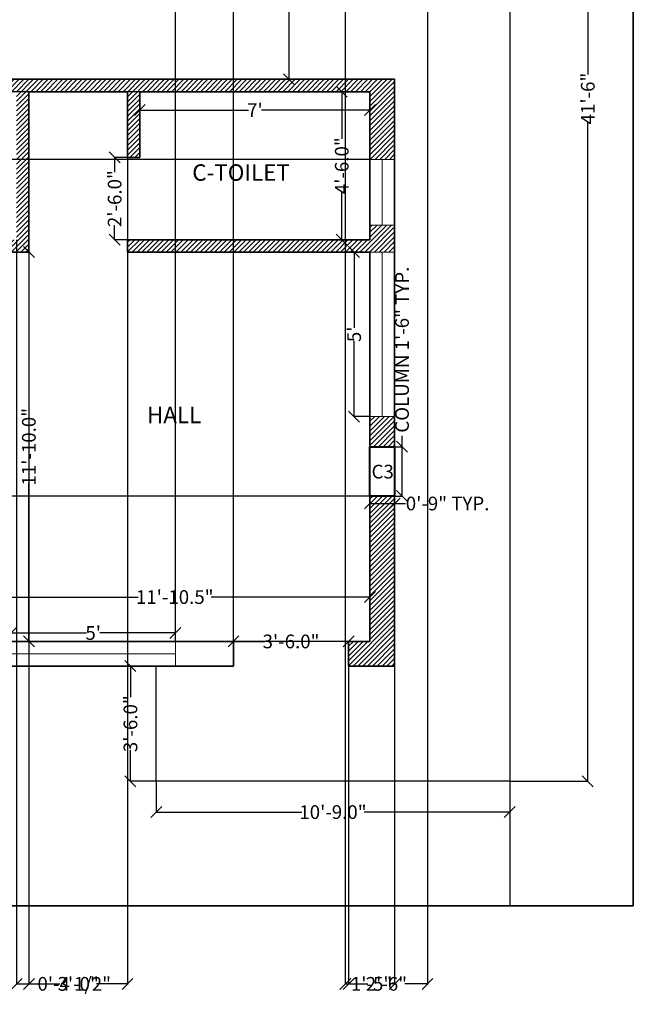
# Model space of a CAD drawing. Units: inches. Extents: x 72 to 538, y -43 to 598.
# Tile 2 of 4: x 314 to 538, y -43 to 316. Entities that reach past the tile are written whole.
import ezdxf

# ---------------------------------------------------------------- set-up
doc = ezdxf.new("R2010")
doc.units = ezdxf.units.IN
doc.header["$MEASUREMENT"] = 0
for name, color, linetype, lineweight in [('A-ANNO-DIMS', 2, 'Continuous', 18), ('A-ANNO-TEXT', 6, 'Continuous', 18), ('A-ANNO-TTLB', 7, 'Continuous', 35), ('A-AREA-IDEN', 7, 'Continuous', 25), ('A-COLS', 6, 'Continuous', 40), ('A-GLAZ', 4, 'Continuous', 18), ('A-WALL', 7, 'Continuous', 35), ('C-SITE', 7, 'Continuous', 25)]:
    doc.layers.add(name, color=color, linetype=linetype, lineweight=lineweight)
doc.layers.add('A-WALL-PATT', color=30, linetype='Continuous', lineweight=13, true_color=0xf26722)
doc.styles.get("Standard").update_dxf_attribs({"font": 'arial.ttf'})
doc.dimstyles.get("Standard").update_dxf_attribs({"dimtxt": 5, "dimasz": 4, "dimexe": 0.18, "dimexo": 0.0625, "dimgap": 0.09, "dimtad": 0, "dimdec": 1, "dimzin": 0, "dimdsep": 46, "dimlunit": 3, "dimtxsty": 'Standard', "dimblk": 'OBLIQUE', "dimcen": 0.09, "dimadec": 0, "dimazin": 0, "dimtfac": 1, "dimtdec": 1, "dimtofl": 0, "dimtmove": 0, "dimatfit": 3, "dimfxl": 1, "dimtolj": 1, "dimtzin": 0, "dimarcsym": 0})

# ---------------------------------------------------------------- blocks, each defined once
blk = doc.blocks.new('_Oblique')
at = {"color": 0, "linetype": 'ByBlock', "lineweight": -2}
blk.add_line((-0.5, -0.5), (0.5, 0.5), dxfattribs=at)
blk = doc.blocks.new('*D20')
at = {"layer": 'A-ANNO-DIMS', "color": 0, "lineweight": -2, "transparency": 16777216}
for p, q in [((317.13, 231.12), (317.13, 173.42)), ((317.19, 231.12), (317.31, 231.12)), ((317.13, 89.12), (317.13, 146.82)), ((317.19, 89.12), (317.31, 89.12))]:
    blk.add_line(p, q, dxfattribs=at)
at = {"layer": 'Defpoints', "color": 0, "transparency": 16777216}
for p in [(317.13, 231.12), (317.13, 89.12), (317.13, 89.12)]:
    blk.add_point(p, dxfattribs=at)
at = {"layer": 'A-ANNO-DIMS', "color": 0, "lineweight": -2, "transparency": 16777216, "xscale": 4, "yscale": 4, "zscale": 4}
for p, rotation in [((317.13, 231.12), 90), ((317.13, 89.12), 270)]:
    blk.add_blockref('_Oblique', p, dxfattribs=dict(at, rotation=rotation))
at = {"layer": 'A-ANNO-DIMS', "color": 0, "transparency": 16777216, "insert": (317.13, 160.12), "char_height": 5, "attachment_point": 5, "rotation": 90}
blk.add_mtext('\\A1;11\'-10.0"', dxfattribs=at)
blk = doc.blocks.new('*D21')
at = {"layer": 'A-ANNO-DIMS', "color": 0, "lineweight": -2, "transparency": 16777216}
for p, q in [((299.13, 113.52), (299.13, 105.13)), ((441.63, 113.52), (441.63, 105.13)), ((299.13, 105.31), (357.08, 105.31)), ((441.63, 105.31), (383.68, 105.31))]:
    blk.add_line(p, q, dxfattribs=at)
at = {"layer": 'Defpoints', "color": 0, "transparency": 16777216}
for p in [(299.13, 113.59), (441.63, 113.59), (441.63, 105.31)]:
    blk.add_point(p, dxfattribs=at)
at = {"layer": 'A-ANNO-DIMS', "color": 0, "lineweight": -2, "transparency": 16777216, "xscale": 4, "yscale": 4, "zscale": 4, "rotation": 180}
blk.add_blockref('_Oblique', (299.13, 105.31), dxfattribs=at)
at = {"layer": 'A-ANNO-DIMS', "color": 0, "lineweight": -2, "transparency": 16777216, "xscale": 4, "yscale": 4, "zscale": 4}
blk.add_blockref('_Oblique', (441.63, 105.31), dxfattribs=at)
at = {"layer": 'A-ANNO-DIMS', "color": 0, "transparency": 16777216, "insert": (370.38, 105.31), "char_height": 5, "attachment_point": 5}
blk.add_mtext('\\A1;11\'-10.5"', dxfattribs=at)
blk = doc.blocks.new('*D22')
at = {"layer": 'A-ANNO-DIMS', "color": 0, "lineweight": -2, "transparency": 16777216}
for p, q in [((441.57, 231.12), (435.66, 231.12)), ((435.84, 231.12), (435.84, 203.51)), ((435.84, 171.12), (435.84, 198.73)), ((441.57, 171.12), (435.66, 171.12))]:
    blk.add_line(p, q, dxfattribs=at)
at = {"layer": 'Defpoints', "color": 0, "transparency": 16777216}
for p in [(441.63, 231.12), (435.84, 171.12), (441.63, 171.12)]:
    blk.add_point(p, dxfattribs=at)
at = {"layer": 'A-ANNO-DIMS', "color": 0, "lineweight": -2, "transparency": 16777216, "xscale": 4, "yscale": 4, "zscale": 4}
for p, rotation in [((435.84, 231.12), 90), ((435.84, 171.12), 270)]:
    blk.add_blockref('_Oblique', p, dxfattribs=dict(at, rotation=rotation))
at = {"layer": 'A-ANNO-DIMS', "color": 0, "transparency": 16777216, "insert": (435.84, 201.12), "char_height": 5, "attachment_point": 5, "rotation": 90}
blk.add_mtext("\\A1;5'", dxfattribs=at)
blk = doc.blocks.new('*D23')
at = {"layer": 'A-ANNO-DIMS', "color": 0, "lineweight": -2, "transparency": 16777216}
for p, q in [((353.07, 265.62), (348.26, 265.62)), ((348.44, 265.62), (348.44, 260.31)), ((348.44, 235.62), (348.44, 240.93)), ((353.07, 235.62), (348.26, 235.62))]:
    blk.add_line(p, q, dxfattribs=at)
at = {"layer": 'Defpoints', "color": 0, "transparency": 16777216}
for p in [(348.44, 265.62), (353.13, 265.62), (353.13, 235.62)]:
    blk.add_point(p, dxfattribs=at)
at = {"layer": 'A-ANNO-DIMS', "color": 0, "lineweight": -2, "transparency": 16777216, "xscale": 4, "yscale": 4, "zscale": 4}
for p, rotation in [((348.44, 265.62), 90), ((348.44, 235.62), 270)]:
    blk.add_blockref('_Oblique', p, dxfattribs=dict(at, rotation=rotation))
at = {"layer": 'A-ANNO-DIMS', "color": 0, "transparency": 16777216, "insert": (348.44, 250.62), "char_height": 5, "attachment_point": 5, "rotation": 90}
blk.add_mtext('\\A1;2\'-6.0"', dxfattribs=at)
blk = doc.blocks.new('*D24')
at = {"layer": 'A-ANNO-DIMS', "color": 0, "lineweight": -2, "transparency": 16777216}
for p, q in [((357.63, 289.56), (357.63, 282.73)), ((441.63, 289.56), (441.63, 282.73)), ((357.63, 282.91), (397.26, 282.91)), ((441.63, 282.91), (402, 282.91))]:
    blk.add_line(p, q, dxfattribs=at)
at = {"layer": 'Defpoints', "color": 0, "transparency": 16777216}
for p in [(357.63, 289.62), (441.63, 289.62), (441.63, 282.91)]:
    blk.add_point(p, dxfattribs=at)
at = {"layer": 'A-ANNO-DIMS', "color": 0, "lineweight": -2, "transparency": 16777216, "xscale": 4, "yscale": 4, "zscale": 4, "rotation": 180}
blk.add_blockref('_Oblique', (357.63, 282.91), dxfattribs=at)
at = {"layer": 'A-ANNO-DIMS', "color": 0, "lineweight": -2, "transparency": 16777216, "xscale": 4, "yscale": 4, "zscale": 4}
blk.add_blockref('_Oblique', (441.63, 282.91), dxfattribs=at)
at = {"layer": 'A-ANNO-DIMS', "color": 0, "transparency": 16777216, "insert": (399.63, 282.91), "char_height": 5, "attachment_point": 5}
blk.add_mtext("\\A1;7'", dxfattribs=at)
blk = doc.blocks.new('*D25')
at = {"layer": 'A-ANNO-DIMS', "color": 0, "lineweight": -2, "transparency": 16777216}
for p, q in [((441.57, 289.62), (431.16, 289.62)), ((431.34, 289.62), (431.34, 272.37)), ((431.34, 235.62), (431.34, 252.87)), ((441.57, 235.62), (431.16, 235.62))]:
    blk.add_line(p, q, dxfattribs=at)
at = {"layer": 'Defpoints', "color": 0, "transparency": 16777216}
for p in [(441.63, 289.62), (431.34, 235.62), (441.63, 235.62)]:
    blk.add_point(p, dxfattribs=at)
at = {"layer": 'A-ANNO-DIMS', "color": 0, "lineweight": -2, "transparency": 16777216, "xscale": 4, "yscale": 4, "zscale": 4}
for p, rotation in [((431.34, 289.62), 90), ((431.34, 235.62), 270)]:
    blk.add_blockref('_Oblique', p, dxfattribs=dict(at, rotation=rotation))
at = {"layer": 'A-ANNO-DIMS', "color": 0, "transparency": 16777216, "insert": (431.34, 262.62), "char_height": 5, "attachment_point": 5, "rotation": 90}
blk.add_mtext('\\A1;4\'-6.0"', dxfattribs=at)
blk = doc.blocks.new('*D27')
at = {"layer": 'A-ANNO-DIMS', "color": 0, "lineweight": -2, "transparency": 16777216}
for p, q in [((423.57, 468.62), (411.92, 468.62)), ((412.1, 468.62), (412.1, 392.73)), ((412.1, 294.12), (412.1, 370.01)), ((423.57, 294.12), (411.92, 294.12))]:
    blk.add_line(p, q, dxfattribs=at)
at = {"layer": 'Defpoints', "color": 0, "transparency": 16777216}
for p in [(423.63, 468.62), (412.1, 294.12), (423.63, 294.12)]:
    blk.add_point(p, dxfattribs=at)
at = {"layer": 'A-ANNO-DIMS', "color": 0, "lineweight": -2, "transparency": 16777216, "xscale": 4, "yscale": 4, "zscale": 4}
for p, rotation in [((412.1, 468.62), 90), ((412.1, 294.12), 270)]:
    blk.add_blockref('_Oblique', p, dxfattribs=dict(at, rotation=rotation))
at = {"layer": 'A-ANNO-DIMS', "color": 0, "transparency": 16777216, "insert": (412.1, 381.37), "char_height": 5, "attachment_point": 5, "rotation": 90}
blk.add_mtext('\\A1;14\'-6.5"', dxfattribs=at)
blk = doc.blocks.new('*D33')
at = {"layer": 'A-ANNO-DIMS', "color": 0, "lineweight": -2, "transparency": 16777216}
for p, q in [((363.57, 80.12), (354.03, 80.12)), ((354.21, 80.12), (354.21, 68.77)), ((354.21, 38.12), (354.21, 49.47)), ((363.57, 38.12), (354.03, 38.12))]:
    blk.add_line(p, q, dxfattribs=at)
at = {"layer": 'Defpoints', "color": 0, "transparency": 16777216}
for p in [(363.63, 80.12), (354.21, 38.12), (363.63, 38.12)]:
    blk.add_point(p, dxfattribs=at)
at = {"layer": 'A-ANNO-DIMS', "color": 0, "lineweight": -2, "transparency": 16777216, "xscale": 4, "yscale": 4, "zscale": 4}
for p, rotation in [((354.21, 80.12), 90), ((354.21, 38.12), 270)]:
    blk.add_blockref('_Oblique', p, dxfattribs=dict(at, rotation=rotation))
at = {"layer": 'A-ANNO-DIMS', "color": 0, "transparency": 16777216, "insert": (354.21, 59.12), "char_height": 5, "attachment_point": 5, "rotation": 90}
blk.add_mtext('\\A1;3\'-6.0"', dxfattribs=at)
blk = doc.blocks.new('*D34')
at = {"layer": 'A-ANNO-DIMS', "color": 0, "lineweight": -2, "transparency": 16777216}
for p, q in [((363.63, 38.06), (363.63, 26.71)), ((492.63, 38.06), (492.63, 26.71)), ((363.63, 26.89), (416.77, 26.89)), ((492.63, 26.89), (439.48, 26.89))]:
    blk.add_line(p, q, dxfattribs=at)
at = {"layer": 'Defpoints', "color": 0, "transparency": 16777216}
for p in [(363.63, 38.12), (492.63, 38.12), (492.63, 26.89)]:
    blk.add_point(p, dxfattribs=at)
at = {"layer": 'A-ANNO-DIMS', "color": 0, "lineweight": -2, "transparency": 16777216, "xscale": 4, "yscale": 4, "zscale": 4, "rotation": 180}
blk.add_blockref('_Oblique', (363.63, 26.89), dxfattribs=at)
at = {"layer": 'A-ANNO-DIMS', "color": 0, "lineweight": -2, "transparency": 16777216, "xscale": 4, "yscale": 4, "zscale": 4}
blk.add_blockref('_Oblique', (492.63, 26.89), dxfattribs=at)
at = {"layer": 'A-ANNO-DIMS', "color": 0, "transparency": 16777216, "insert": (428.13, 26.89), "char_height": 5, "attachment_point": 5}
blk.add_mtext('\\A1;10\'-9.0"', dxfattribs=at)
blk = doc.blocks.new('*D35')
at = {"layer": 'A-ANNO-DIMS', "color": 0, "lineweight": -2, "transparency": 16777216}
for p, q in [((391.82, 89.12), (403.17, 89.12)), ((391.82, 89.06), (391.82, 88.94)), ((433.82, 89.12), (422.47, 89.12)), ((433.82, 89.18), (433.82, 89.3))]:
    blk.add_line(p, q, dxfattribs=at)
at = {"layer": 'Defpoints', "color": 0, "transparency": 16777216}
for p in [(391.82, 89.12), (433.82, 89.12), (433.82, 89.12)]:
    blk.add_point(p, dxfattribs=at)
at = {"layer": 'A-ANNO-DIMS', "color": 0, "lineweight": -2, "transparency": 16777216, "xscale": 4, "yscale": 4, "zscale": 4, "rotation": 180}
blk.add_blockref('_Oblique', (391.82, 89.12), dxfattribs=at)
at = {"layer": 'A-ANNO-DIMS', "color": 0, "lineweight": -2, "transparency": 16777216, "xscale": 4, "yscale": 4, "zscale": 4}
blk.add_blockref('_Oblique', (433.82, 89.12), dxfattribs=at)
at = {"layer": 'A-ANNO-DIMS', "color": 0, "transparency": 16777216, "insert": (412.82, 89.12), "char_height": 5, "attachment_point": 5}
blk.add_mtext('\\A1;3\'-6.0"', dxfattribs=at)
blk = doc.blocks.new('*D36')
at = {"layer": 'A-ANNO-DIMS', "color": 0, "lineweight": -2, "transparency": 16777216}
for p, q in [((310.61, 89.18), (310.61, 92.39)), ((310.61, 92.21), (338.22, 92.21)), ((370.61, 92.21), (343, 92.21)), ((370.61, 89.18), (370.61, 92.39))]:
    blk.add_line(p, q, dxfattribs=at)
at = {"layer": 'Defpoints', "color": 0, "transparency": 16777216}
for p in [(370.61, 92.21), (310.61, 89.12), (370.61, 89.12)]:
    blk.add_point(p, dxfattribs=at)
at = {"layer": 'A-ANNO-DIMS', "color": 0, "lineweight": -2, "transparency": 16777216, "xscale": 4, "yscale": 4, "zscale": 4, "rotation": 180}
blk.add_blockref('_Oblique', (310.61, 92.21), dxfattribs=at)
at = {"layer": 'A-ANNO-DIMS', "color": 0, "lineweight": -2, "transparency": 16777216, "xscale": 4, "yscale": 4, "zscale": 4}
blk.add_blockref('_Oblique', (370.61, 92.21), dxfattribs=at)
at = {"layer": 'A-ANNO-DIMS', "color": 0, "transparency": 16777216, "insert": (340.61, 92.21), "char_height": 5, "attachment_point": 5}
blk.add_mtext("\\A1;5'", dxfattribs=at)
blk = doc.blocks.new('COL-9X18')
for p, q in [((0, 18), (9, 18)), ((0, 0), (0, 18)), ((9, 18), (9, 0)), ((9, 0), (0, 0))]:
    blk.add_line(p, q)
blk = doc.blocks.new('WIN-60')
for p, q in [((0, 9), (0, 0)), ((60, 9), (60, 0)), ((0, 4.5), (60, 4.5))]:
    blk.add_line(p, q)
blk = doc.blocks.new('WIN-24')
for p, q in [((0, 0), (0, 9)), ((24, 0), (24, 9)), ((0, 4.5), (24, 4.5))]:
    blk.add_line(p, q)
blk = doc.blocks.new('*D44')
at = {"layer": 'A-ANNO-DIMS', "color": 0, "lineweight": -2, "transparency": 16777216}
for p, q in [((453.33, 160.12), (453.33, 164.12)), ((450.69, 160.12), (453.51, 160.12)), ((453.33, 142.12), (453.33, 160.12)), ((450.69, 142.12), (453.51, 142.12))]:
    blk.add_line(p, q, dxfattribs=at)
at = {"layer": 'Defpoints', "color": 0, "transparency": 16777216}
for p in [(450.63, 160.12), (453.33, 160.12), (450.63, 142.12)]:
    blk.add_point(p, dxfattribs=at)
at = {"layer": 'A-ANNO-DIMS', "color": 0, "lineweight": -2, "transparency": 16777216, "xscale": 4, "yscale": 4, "zscale": 4}
for p, rotation in [((453.33, 160.12), 90), ((453.33, 142.12), 270)]:
    blk.add_blockref('_Oblique', p, dxfattribs=dict(at, rotation=rotation))
at = {"layer": 'A-ANNO-DIMS', "color": 0, "transparency": 16777216, "insert": (453.33, 195.52), "char_height": 5, "attachment_point": 5, "rotation": 90}
blk.add_mtext('\\A1;COLUMN 1\'-6" TYP.', dxfattribs=at)
blk = doc.blocks.new('*D45')
at = {"layer": 'A-ANNO-DIMS', "color": 0, "lineweight": -2, "transparency": 16777216}
for p, q in [((441.63, 142.06), (441.63, 139.24)), ((450.63, 142.06), (450.63, 139.24)), ((441.63, 139.42), (450.63, 139.42)), ((450.63, 139.42), (454.63, 139.42))]:
    blk.add_line(p, q, dxfattribs=at)
at = {"layer": 'Defpoints', "color": 0, "transparency": 16777216}
for p in [(441.63, 142.12), (450.63, 142.12), (450.63, 139.42)]:
    blk.add_point(p, dxfattribs=at)
at = {"layer": 'A-ANNO-DIMS', "color": 0, "lineweight": -2, "transparency": 16777216, "xscale": 4, "yscale": 4, "zscale": 4, "rotation": 180}
blk.add_blockref('_Oblique', (441.63, 139.42), dxfattribs=at)
at = {"layer": 'A-ANNO-DIMS', "color": 0, "lineweight": -2, "transparency": 16777216, "xscale": 4, "yscale": 4, "zscale": 4}
blk.add_blockref('_Oblique', (450.63, 139.42), dxfattribs=at)
at = {"layer": 'A-ANNO-DIMS', "color": 0, "transparency": 16777216, "insert": (469.96, 139.42), "char_height": 5, "attachment_point": 5}
blk.add_mtext('\\A1;0\'-9" TYP.', dxfattribs=at)
blk = doc.blocks.new('*D53')
at = {"layer": 'A-ANNO-DIMS', "color": 0, "lineweight": -2, "transparency": 16777216}
for p, q in [((492.69, 536.12), (521.31, 536.12)), ((521.13, 536.12), (521.13, 295.9)), ((521.13, 38.12), (521.13, 278.34)), ((492.69, 38.12), (521.31, 38.12))]:
    blk.add_line(p, q, dxfattribs=at)
at = {"layer": 'Defpoints', "color": 0, "transparency": 16777216}
for p in [(492.63, 536.12), (521.13, 536.12), (492.63, 38.12)]:
    blk.add_point(p, dxfattribs=at)
at = {"layer": 'A-ANNO-DIMS', "color": 0, "lineweight": -2, "transparency": 16777216, "xscale": 4, "yscale": 4, "zscale": 4}
for p, rotation in [((521.13, 536.12), 90), ((521.13, 38.12), 270)]:
    blk.add_blockref('_Oblique', p, dxfattribs=dict(at, rotation=rotation))
at = {"layer": 'A-ANNO-DIMS', "color": 0, "transparency": 16777216, "insert": (521.13, 287.12), "char_height": 5, "attachment_point": 5, "rotation": 90}
blk.add_mtext('\\A1;41\'-6"', dxfattribs=at)
blk = doc.blocks.new('*D54')
at = {"layer": 'A-ANNO-DIMS', "color": 0, "lineweight": -2, "transparency": 16777216}
for p, q in [((432.63, 381.06), (432.63, -35.94)), ((462.63, 381.06), (462.63, -35.94)), ((432.63, -35.76), (440.85, -35.76)), ((462.63, -35.76), (454.41, -35.76))]:
    blk.add_line(p, q, dxfattribs=at)
at = {"layer": 'Defpoints', "color": 0, "transparency": 16777216}
for p in [(432.63, 381.12), (462.63, 381.12), (462.63, -35.76)]:
    blk.add_point(p, dxfattribs=at)
at = {"layer": 'A-ANNO-DIMS', "color": 0, "lineweight": -2, "transparency": 16777216, "xscale": 4, "yscale": 4, "zscale": 4, "rotation": 180}
blk.add_blockref('_Oblique', (432.63, -35.76), dxfattribs=at)
at = {"layer": 'A-ANNO-DIMS', "color": 0, "lineweight": -2, "transparency": 16777216, "xscale": 4, "yscale": 4, "zscale": 4}
blk.add_blockref('_Oblique', (462.63, -35.76), dxfattribs=at)
at = {"layer": 'A-ANNO-DIMS', "color": 0, "transparency": 16777216, "insert": (447.63, -35.76), "char_height": 5, "attachment_point": 5}
blk.add_mtext('\\A1;2\'-6"', dxfattribs=at)
blk = doc.blocks.new('*D60')
at = {"layer": 'A-ANNO-DIMS', "color": 0, "lineweight": -2, "transparency": 16777216}
for p, q in [((370.61, 89.18), (370.61, 588.8)), ((370.61, 588.62), (374.71, 588.62)), ((391.82, 588.62), (387.71, 588.62)), ((391.82, 89.18), (391.82, 588.8))]:
    blk.add_line(p, q, dxfattribs=at)
at = {"layer": 'Defpoints', "color": 0, "transparency": 16777216}
for p in [(391.82, 588.62), (370.61, 89.12), (391.82, 89.12)]:
    blk.add_point(p, dxfattribs=at)
at = {"layer": 'A-ANNO-DIMS', "color": 0, "lineweight": -2, "transparency": 16777216, "xscale": 4, "yscale": 4, "zscale": 4, "rotation": 180}
blk.add_blockref('_Oblique', (370.61, 588.62), dxfattribs=at)
at = {"layer": 'A-ANNO-DIMS', "color": 0, "lineweight": -2, "transparency": 16777216, "xscale": 4, "yscale": 4, "zscale": 4}
blk.add_blockref('_Oblique', (391.82, 588.62), dxfattribs=at)
at = {"layer": 'A-ANNO-DIMS', "color": 0, "transparency": 16777216, "insert": (381.21, 588.62), "char_height": 5, "attachment_point": 5}
blk.add_mtext('\\A1;1\'-9"', dxfattribs=at)
blk = doc.blocks.new('*D61')
at = {"layer": 'A-ANNO-DIMS', "color": 0, "lineweight": -2, "transparency": 16777216}
for p, q in [((433.82, 80.06), (433.82, -35.94)), ((450.63, 80.06), (450.63, -35.94)), ((433.82, -35.76), (435.72, -35.76)), ((450.63, -35.76), (448.72, -35.76))]:
    blk.add_line(p, q, dxfattribs=at)
at = {"layer": 'Defpoints', "color": 0, "transparency": 16777216}
for p in [(433.82, 80.12), (450.63, 80.12), (450.63, -35.76)]:
    blk.add_point(p, dxfattribs=at)
at = {"layer": 'A-ANNO-DIMS', "color": 0, "lineweight": -2, "transparency": 16777216, "xscale": 4, "yscale": 4, "zscale": 4, "rotation": 180}
blk.add_blockref('_Oblique', (433.82, -35.76), dxfattribs=at)
at = {"layer": 'A-ANNO-DIMS', "color": 0, "lineweight": -2, "transparency": 16777216, "xscale": 4, "yscale": 4, "zscale": 4}
blk.add_blockref('_Oblique', (450.63, -35.76), dxfattribs=at)
at = {"layer": 'A-ANNO-DIMS', "color": 0, "transparency": 16777216, "insert": (442.22, -35.76), "char_height": 5, "attachment_point": 5}
blk.add_mtext('\\A1;1\'-5"', dxfattribs=at)
blk = doc.blocks.new('*D64')
at = {"layer": 'A-ANNO-DIMS', "color": 0, "lineweight": -2, "transparency": 16777216}
for p, q in [((317.13, 289.56), (317.13, -35.94)), ((353.13, 289.56), (353.13, -35.94)), ((317.13, -35.76), (328.4, -35.76)), ((353.13, -35.76), (341.86, -35.76))]:
    blk.add_line(p, q, dxfattribs=at)
at = {"layer": 'Defpoints', "color": 0, "transparency": 16777216}
for p in [(317.13, 289.62), (353.13, 289.62), (353.13, -35.76)]:
    blk.add_point(p, dxfattribs=at)
at = {"layer": 'A-ANNO-DIMS', "color": 0, "lineweight": -2, "transparency": 16777216, "xscale": 4, "yscale": 4, "zscale": 4, "rotation": 180}
blk.add_blockref('_Oblique', (317.13, -35.76), dxfattribs=at)
at = {"layer": 'A-ANNO-DIMS', "color": 0, "lineweight": -2, "transparency": 16777216, "xscale": 4, "yscale": 4, "zscale": 4}
blk.add_blockref('_Oblique', (353.13, -35.76), dxfattribs=at)
at = {"layer": 'A-ANNO-DIMS', "color": 0, "transparency": 16777216, "insert": (335.13, -35.76), "char_height": 5, "attachment_point": 5}
blk.add_mtext('\\A1;3\'-0"', dxfattribs=at)
blk = doc.blocks.new('*D65')
at = {"layer": 'A-ANNO-DIMS', "color": 0, "lineweight": -2, "transparency": 16777216}
for p, q in [((312.63, 235.56), (312.63, -35.94)), ((317.13, 231.06), (317.13, -35.94)), ((312.63, -35.76), (317.13, -35.76)), ((317.13, -35.76), (321.13, -35.76))]:
    blk.add_line(p, q, dxfattribs=at)
at = {"layer": 'Defpoints', "color": 0, "transparency": 16777216}
for p in [(312.63, 235.62), (317.13, 231.12), (317.13, -35.76)]:
    blk.add_point(p, dxfattribs=at)
at = {"layer": 'A-ANNO-DIMS', "color": 0, "lineweight": -2, "transparency": 16777216, "xscale": 4, "yscale": 4, "zscale": 4, "rotation": 180}
blk.add_blockref('_Oblique', (312.63, -35.76), dxfattribs=at)
at = {"layer": 'A-ANNO-DIMS', "color": 0, "lineweight": -2, "transparency": 16777216, "xscale": 4, "yscale": 4, "zscale": 4}
blk.add_blockref('_Oblique', (317.13, -35.76), dxfattribs=at)
at = {"layer": 'A-ANNO-DIMS', "color": 0, "transparency": 16777216, "insert": (333.69, -35.76), "char_height": 5, "attachment_point": 5}
blk.add_mtext('\\A1;0\'-4 1/2"', dxfattribs=at)
blk = doc.blocks.new('*D66')
at = {"layer": 'A-ANNO-DIMS', "color": 0, "lineweight": -2, "transparency": 16777216}
for p, q in [((441.57, 289.62), (103.95, 289.62)), ((104.13, 289.62), (104.13, 264.93)), ((441.57, 264.93), (103.95, 264.93)), ((104.13, 264.93), (104.13, 260.93))]:
    blk.add_line(p, q, dxfattribs=at)
at = {"layer": 'Defpoints', "color": 0, "transparency": 16777216}
for p in [(441.63, 289.62), (104.13, 264.93), (441.63, 264.93)]:
    blk.add_point(p, dxfattribs=at)
at = {"layer": 'A-ANNO-DIMS', "color": 0, "lineweight": -2, "transparency": 16777216, "xscale": 4, "yscale": 4, "zscale": 4}
for p, rotation in [((104.13, 289.62), 90), ((104.13, 264.93), 270)]:
    blk.add_blockref('_Oblique', p, dxfattribs=dict(at, rotation=rotation))
at = {"layer": 'A-ANNO-DIMS', "color": 0, "transparency": 16777216, "insert": (104.13, 248.33), "char_height": 5, "attachment_point": 5, "rotation": 90}
blk.add_mtext('\\A1;2\'-0 1/2"', dxfattribs=at)
blk = doc.blocks.new('*D69')
at = {"layer": 'A-ANNO-DIMS', "color": 0, "lineweight": -2, "transparency": 16777216}
for p, q in [((441.57, 142.12), (103.95, 142.12)), ((104.13, 142.12), (104.13, 122.46)), ((104.13, 89.12), (104.13, 108.78)), ((441.57, 89.12), (103.95, 89.12))]:
    blk.add_line(p, q, dxfattribs=at)
at = {"layer": 'Defpoints', "color": 0, "transparency": 16777216}
for p in [(441.63, 142.12), (104.13, 89.12), (441.63, 89.12)]:
    blk.add_point(p, dxfattribs=at)
at = {"layer": 'A-ANNO-DIMS', "color": 0, "lineweight": -2, "transparency": 16777216, "xscale": 4, "yscale": 4, "zscale": 4}
for p, rotation in [((104.13, 142.12), 90), ((104.13, 89.12), 270)]:
    blk.add_blockref('_Oblique', p, dxfattribs=dict(at, rotation=rotation))
at = {"layer": 'A-ANNO-DIMS', "color": 0, "transparency": 16777216, "insert": (104.13, 115.62), "char_height": 5, "attachment_point": 5, "rotation": 90}
blk.add_mtext('\\A1;4\'-5"', dxfattribs=at)

msp = doc.modelspace()

# ---------------------------------------------------------------- hatches: boundary and pattern name
at = {"layer": 'A-WALL-PATT'}
h = msp.add_hatch(dxfattribs=at)
h.set_pattern_fill('ANSI31', color=256, scale=10)
h.paths.add_polyline_path([(204.03, 536.12), (165.63, 536.12), (165.63, 527.12), (204.03, 527.12)])
h.paths.add_polyline_path([(165.63, 487.18), (165.63, 518.12), (156.63, 518.12), (156.63, 487.18)])
h.paths.add_polyline_path([(374.85, 253.74), (416.04, 253.74), (416.04, 266.11), (374.85, 266.11)], flags=9)
h.paths.add_polyline_path([(358.05, 165.41), (382.02, 165.41), (382.02, 177.78), (358.05, 177.78)], flags=9)
h.paths.add_polyline_path([(258.82, 340.82), (290.25, 340.82), (290.25, 353.18), (258.82, 353.18)], flags=9)
h.paths.add_polyline_path([(190.8, 385.39), (230.59, 385.39), (230.59, 397.75), (190.8, 397.75)], flags=9)
h.paths.add_polyline_path([(259.76, 122.35), (291.18, 122.35), (291.18, 134.72), (259.76, 134.72)], flags=9)
h.paths.add_polyline_path([(192.66, 147.9), (232.45, 147.9), (232.45, 160.26), (192.66, 160.26)], flags=9)
h.paths.add_polyline_path([(197.84, 250.21), (246.48, 250.21), (246.48, 262.58), (197.84, 262.58)], flags=9)
h.paths.add_polyline_path([(329.22, 365.75), (353.18, 365.75), (353.18, 378.11), (329.22, 378.11)], flags=9)
h.paths.add_polyline_path([(351.21, 489.41), (392.39, 489.41), (392.39, 501.77), (351.21, 501.77)], flags=9)
h.paths.add_polyline_path([(193.31, 469.76), (241.95, 469.76), (241.95, 482.12), (193.31, 482.12)], flags=9)
h.paths.add_polyline_path([(262.62, 413.67), (274.04, 413.67), (274.04, 423.97), (262.62, 423.97)], flags=9)
h.paths.add_polyline_path([(155.57, 341.76), (167, 341.76), (167, 352.06), (155.57, 352.06)], flags=9)
h.paths.add_polyline_path([(155.43, 129.83), (166.86, 129.83), (166.86, 140.14), (155.43, 140.14)], flags=9)
h.paths.add_polyline_path([(293.27, 137.19), (304.7, 137.19), (304.7, 147.49), (293.27, 147.49)], flags=9)
h.paths.add_polyline_path([(440.6, 145.74), (452.03, 145.74), (452.03, 156.04), (440.6, 156.04)], flags=9)
h.paths.add_polyline_path([(422.43, 340.03), (433.86, 340.03), (433.86, 350.33), (422.43, 350.33)], flags=9)
h.paths.add_polyline_path([(155.47, 520.54), (166.9, 520.54), (166.9, 530.84), (155.47, 530.84)], flags=9)
h.paths.add_polyline_path([(348.1, 449.93), (374.22, 449.93), (374.22, 460.24), (348.1, 460.24)], flags=9)
h.paths.add_polyline_path([(417.29, 368.09), (417.29, 394.21), (406.99, 394.21), (406.99, 368.09)], flags=9)
h.paths.add_polyline_path([(422.51, 520.96), (433.94, 520.96), (433.94, 531.26), (422.51, 531.26)], flags=9)
h.paths.add_polyline_path([(284.05, 526.61), (295.48, 526.61), (295.48, 536.92), (284.05, 536.92)], flags=9)
h = msp.add_hatch(dxfattribs=at)
h.set_pattern_fill('ANSI31', color=256, scale=10)
h.paths.add_polyline_path([(432.63, 468.62), (432.63, 518.12), (423.63, 518.12), (423.63, 473.12), (339.63, 473.12), (335.13, 473.12), (335.13, 468.62), (423.63, 468.62), (423.63, 354.62), (432.63, 354.62)])
h.paths.add_polyline_path([(450.63, 231.12), (450.63, 240.93), (441.63, 240.93), (441.63, 235.62), (357.63, 235.62), (353.13, 235.62), (353.13, 231.12), (441.63, 231.12)])
h.paths.add_polyline_path([(374.85, 253.74), (416.04, 253.74), (416.04, 266.11), (374.85, 266.11)], flags=9)
h.paths.add_polyline_path([(358.05, 165.41), (382.02, 165.41), (382.02, 177.78), (358.05, 177.78)], flags=9)
h.paths.add_polyline_path([(258.82, 340.82), (290.25, 340.82), (290.25, 353.18), (258.82, 353.18)], flags=9)
h.paths.add_polyline_path([(190.8, 385.39), (230.59, 385.39), (230.59, 397.75), (190.8, 397.75)], flags=9)
h.paths.add_polyline_path([(259.76, 122.35), (291.18, 122.35), (291.18, 134.72), (259.76, 134.72)], flags=9)
h.paths.add_polyline_path([(192.66, 147.9), (232.45, 147.9), (232.45, 160.26), (192.66, 160.26)], flags=9)
h.paths.add_polyline_path([(197.84, 250.21), (246.48, 250.21), (246.48, 262.58), (197.84, 262.58)], flags=9)
h.paths.add_polyline_path([(329.22, 365.75), (353.18, 365.75), (353.18, 378.11), (329.22, 378.11)], flags=9)
h.paths.add_polyline_path([(351.21, 489.41), (392.39, 489.41), (392.39, 501.77), (351.21, 501.77)], flags=25)
h.paths.add_polyline_path([(193.31, 469.76), (241.95, 469.76), (241.95, 482.12), (193.31, 482.12)], flags=9)
h.paths.add_polyline_path([(262.62, 413.67), (274.04, 413.67), (274.04, 423.97), (262.62, 423.97)], flags=9)
h.paths.add_polyline_path([(155.57, 341.76), (167, 341.76), (167, 352.06), (155.57, 352.06)], flags=9)
h.paths.add_polyline_path([(155.43, 129.83), (166.86, 129.83), (166.86, 140.14), (155.43, 140.14)], flags=9)
h.paths.add_polyline_path([(293.27, 137.19), (304.7, 137.19), (304.7, 147.49), (293.27, 147.49)], flags=9)
h.paths.add_polyline_path([(440.6, 145.74), (452.03, 145.74), (452.03, 156.04), (440.6, 156.04)], flags=9)
h.paths.add_polyline_path([(422.43, 340.03), (433.86, 340.03), (433.86, 350.33), (422.43, 350.33)], flags=9)
h.paths.add_polyline_path([(422.51, 520.96), (433.94, 520.96), (433.94, 531.26), (422.51, 531.26)], flags=9)
h.paths.add_polyline_path([(284.05, 526.61), (295.48, 526.61), (295.48, 536.92), (284.05, 536.92)], flags=9)
h.paths.add_polyline_path([(155.47, 520.54), (166.9, 520.54), (166.9, 530.84), (155.47, 530.84)], flags=9)
h = msp.add_hatch(dxfattribs=at)
h.set_pattern_fill('ANSI31', color=256, scale=10)
h.paths.add_polyline_path([(165.63, 427.18), (156.63, 427.18), (156.63, 414.62), (165.63, 414.62), (258.91, 414.62), (258.91, 419.12), (165.63, 419.12)])
h.paths.add_polyline_path([(165.63, 378.62), (156.63, 378.62), (156.63, 355.53), (165.63, 355.53)])
h.paths.add_polyline_path([(299.13, 378.12), (290.13, 378.12), (290.13, 373.62), (294.63, 373.62), (294.63, 318.12), (252.63, 318.12), (252.63, 373.62), (257.13, 373.62), (257.13, 378.12), (248.13, 378.12), (248.13, 318.12), (165.63, 318.12), (165.63, 337.53), (156.63, 337.53), (156.63, 294.2), (165.63, 294.2), (165.63, 313.62), (294.63, 313.62), (294.63, 289.62), (312.63, 289.62), (312.63, 235.62), (294.63, 235.62), (294.63, 231.12), (317.13, 231.12), (317.13, 289.62), (353.13, 289.62), (353.13, 265.62), (357.63, 265.62), (357.63, 289.62), (441.63, 289.62), (441.63, 264.93), (450.63, 264.93), (450.63, 294.12), (432.63, 294.12), (299.13, 294.12)])
h.paths.add_polyline_path([(299.13, 195.12), (165.63, 195.12), (165.63, 234.2), (156.63, 234.2), (156.63, 144.66), (165.63, 144.66), (165.63, 190.62), (299.13, 190.62)])
h.paths.add_polyline_path([(165.63, 126.66), (156.63, 126.66), (156.63, 80.12), (212.13, 80.12), (212.13, 89.12), (165.63, 89.12)])
h.paths.add_polyline_path([(310.61, 89.12), (299.13, 89.12), (299.13, 137.87), (294.63, 137.87), (294.63, 89.12), (252.63, 89.12), (252.63, 144.62), (257.13, 144.62), (257.13, 149.12), (248.13, 149.12), (248.13, 89.12), (248.13, 80.12), (310.61, 80.12)])
h.paths.add_polyline_path([(450.63, 142.12), (441.63, 142.12), (441.63, 89.12), (433.82, 89.12), (433.82, 80.12), (450.63, 80.12)])
h.paths.add_polyline_path([(450.63, 171.12), (446.13, 171.12), (441.63, 171.12), (441.63, 160.12), (450.63, 160.12)])
h.paths.add_polyline_path([(281.13, 536.12), (264.03, 536.12), (264.03, 527.12), (281.13, 527.12)])
h.paths.add_polyline_path([(339.63, 536.12), (299.13, 536.12), (299.13, 527.12), (335.13, 527.12), (335.13, 503.12), (339.63, 503.12), (339.63, 527.12)])
h.paths.add_polyline_path([(299.13, 527.12), (294.63, 527.12), (294.63, 455.12), (299.13, 455.12)])
h.paths.add_polyline_path([(492.63, 536.12), (432.63, 536.12), (432.63, 527.12), (492.63, 527.12)])
h.paths.add_polyline_path([(423.63, 536.12), (363.63, 536.12), (363.63, 527.12), (423.63, 527.12)])
h.paths.add_polyline_path([(299.13, 419.12), (276.91, 419.12), (276.91, 414.62), (299.13, 414.62)])

# ---------------------------------------------------------------- linework, layer by layer
at = {"layer": 'A-ANNO-TTLB'}
msp.add_lwpolyline([(72.29, 598.2), (537.75, 598.2), (537.75, -7.26), (72.29, -7.26)], close=True, dxfattribs=at)
at = {"layer": 'A-GLAZ'}
for p, q in [((441.63, 231.12), (441.63, 171.12)), ((446.13, 231.12), (441.63, 231.12)), ((450.63, 171.12), (446.13, 171.12))]:
    msp.add_line(p, q, dxfattribs=at)
at = {"layer": 'A-WALL'}
for p, q in [((299.13, 294.12), (432.63, 294.12)), ((432.63, 294.12), (450.63, 294.12)), ((450.63, 80.12), (450.63, 294.12)), ((317.13, 289.62), (317.13, 231.12)), ((317.13, 289.62), (353.13, 289.62)), ((353.13, 265.62), (353.13, 289.62)), ((357.63, 265.62), (357.63, 289.62)), ((357.63, 289.62), (441.63, 289.62)), ((441.63, 235.62), (441.63, 289.62)), ((353.13, 265.62), (357.63, 265.62)), ((353.13, 235.62), (357.63, 235.62)), ((353.13, 235.62), (353.13, 231.12)), ((357.63, 235.62), (441.63, 235.62)), ((294.63, 231.12), (317.13, 231.12)), ((353.13, 231.12), (441.63, 231.12)), ((441.63, 89.12), (441.63, 231.12)), ((391.82, 89.12), (299.13, 89.12)), ((391.82, 89.12), (391.82, 80.12)), ((441.63, 89.12), (433.82, 89.12)), ((433.82, 89.12), (433.82, 80.12)), ((391.82, 80.12), (156.63, 80.12)), ((450.63, 80.12), (433.82, 80.12))]:
    msp.add_line(p, q, dxfattribs=at)
at = {"layer": 'C-SITE'}
for p, q in [((492.63, 560.12), (492.63, -7.26)), ((363.63, 38.12), (363.63, 80.12)), ((492.63, 80.12), (492.63, 38.12)), ((492.63, 38.12), (363.63, 38.12))]:
    msp.add_line(p, q, dxfattribs=at)

# ---------------------------------------------------------------- block references
at = {"layer": 'A-COLS'}
msp.add_blockref('COL-9X18', (441.63, 142.12), dxfattribs=at)
at = {"layer": 'A-GLAZ'}
for name, p, rotation in [('WIN-24', (450.63, 240.93), 90.00000000000031), ('WIN-60', (441.63, 231.12), 269.9999999999997), ('WIN-60', (370.61, 89.12), 180)]:
    msp.add_blockref(name, p, dxfattribs=dict(at, rotation=rotation))

# ---------------------------------------------------------------- texts
at = {"layer": 'A-ANNO-TEXT', "insert": (442.2, 153.55), "char_height": 5, "attachment_point": 1}
msp.add_mtext_dynamic_manual_height_columns('C3', width=12, gutter_width=1, heights=[0], dxfattribs=at)
at = {"layer": 'A-AREA-IDEN', "char_height": 6, "attachment_point": 1}
for s, insert in [('C-TOILET', (376.77, 263.13)), ('HALL', (360.23, 174.69))]:
    msp.add_mtext_dynamic_manual_height_columns(s, width=78.4308, gutter_width=1, heights=[0], dxfattribs=dict(at, insert=insert))

# ---------------------------------------------------------------- dimensions: what is measured, and where the dimension line sits
at = {"layer": 'A-ANNO-DIMS'}
for base, p1, p2, override, picture, middle in [((391.82, 588.62), (370.61, 89.12), (391.82, 89.12), {"dimdec": 1, "dimlfac": 1, "dimrnd": 0, "dimzin": 1, "dimdsep": 46, "dimlunit": 4, "dimfrac": 2}, '*D60', (381.21, 588.62)), ((462.63, -35.76), (432.63, 381.12), (462.63, 381.12), {"dimdec": 1, "dimlfac": 1, "dimrnd": 0, "dimzin": 1, "dimdsep": 46, "dimlunit": 4, "dimfrac": 2}, '*D54', (447.63, -35.76)), ((353.13, -35.76), (317.13, 289.62), (353.13, 289.62), {"dimdec": 1, "dimlfac": 1, "dimrnd": 0, "dimzin": 1, "dimdsep": 46, "dimlunit": 4, "dimfrac": 2}, '*D64', (335.13, -35.76)), ((441.63, 282.91), (357.63, 289.62), (441.63, 289.62), {"dimclrd": 0, "dimclre": 0, "dimclrt": 0}, '*D24', (399.63, 282.91)), ((317.13, -35.76), (312.63, 235.62), (317.13, 231.12), {"dimdec": 1, "dimlfac": 1, "dimrnd": 0, "dimzin": 1, "dimdsep": 46, "dimlunit": 4, "dimfrac": 2}, '*D65', (333.69, -35.76)), ((441.63, 105.31), (299.13, 113.59), (441.63, 113.59), {"dimclrd": 0, "dimclre": 0, "dimclrt": 0}, '*D21', (370.38, 105.31)), ((370.61, 92.21), (310.61, 89.12), (370.61, 89.12), {"dimclrd": 0, "dimclre": 0, "dimclrt": 0}, '*D36', (340.61, 92.21)), ((433.82, 89.12), (391.82, 89.12), (433.82, 89.12), {"dimclrd": 0, "dimclre": 0, "dimclrt": 0}, '*D35', (412.82, 89.12)), ((450.63, -35.76), (433.82, 80.12), (450.63, 80.12), {"dimdec": 1, "dimlfac": 1, "dimrnd": 0, "dimzin": 1, "dimdsep": 46, "dimlunit": 4, "dimfrac": 2}, '*D61', (442.22, -35.76)), ((492.63, 26.89), (363.63, 38.12), (492.63, 38.12), {"dimclrd": 0, "dimclre": 0, "dimclrt": 0}, '*D34', (428.13, 26.89))]:
    dim = msp.add_linear_dim(base=base, p1=p1, p2=p2, dimstyle='Standard', override=override, dxfattribs=at)
    dim.commit()
    dim.dimension.update_dxf_attribs({"geometry": picture, "text_midpoint": middle})
for base, p1, p2, override, picture, middle in [((521.13, 536.12), (492.63, 38.12), (492.63, 536.12), {"dimdec": 1, "dimlfac": 1, "dimrnd": 0, "dimzin": 1, "dimdsep": 46, "dimlunit": 4, "dimfrac": 2}, '*D53', (521.13, 287.12)), ((412.1, 294.12), (423.63, 468.62), (423.63, 294.12), {"dimclrd": 0, "dimclre": 0, "dimclrt": 0}, '*D27', (412.1, 381.37)), ((104.13, 264.93), (441.63, 289.62), (441.63, 264.93), {"dimdec": 1, "dimlfac": 1, "dimrnd": 0, "dimzin": 1, "dimdsep": 46, "dimlunit": 4, "dimfrac": 2}, '*D66', (104.13, 248.33)), ((431.34, 235.62), (441.63, 289.62), (441.63, 235.62), {"dimclrd": 0, "dimclre": 0, "dimclrt": 0}, '*D25', (431.34, 262.62)), ((348.44, 265.62), (353.13, 235.62), (353.13, 265.62), {"dimclrd": 0, "dimclre": 0, "dimclrt": 0}, '*D23', (348.44, 250.62)), ((317.13, 89.12), (317.13, 231.12), (317.13, 89.12), {"dimclrd": 0, "dimclre": 0, "dimclrt": 0}, '*D20', (317.13, 160.12)), ((435.84, 171.12), (441.63, 231.12), (441.63, 171.12), {"dimclrd": 0, "dimclre": 0, "dimclrt": 0}, '*D22', (435.84, 201.12)), ((104.13, 89.12), (441.63, 142.12), (441.63, 89.12), {"dimdec": 1, "dimlfac": 1, "dimrnd": 0, "dimzin": 1, "dimdsep": 46, "dimlunit": 4, "dimfrac": 2}, '*D69', (104.13, 115.62)), ((354.21, 38.12), (363.63, 80.12), (363.63, 38.12), {"dimclrd": 0, "dimclre": 0, "dimclrt": 0}, '*D33', (354.21, 59.12))]:
    dim = msp.add_linear_dim(base=base, p1=p1, p2=p2, angle=90, dimstyle='Standard', override=override, dxfattribs=at)
    dim.commit()
    dim.dimension.update_dxf_attribs({"geometry": picture, "text_midpoint": middle})
dim = msp.add_linear_dim(base=(453.33, 160.12), p1=(450.63, 142.12), p2=(450.63, 160.12), angle=90, text='COLUMN <> TYP.', dimstyle='Standard', override={"dimdec": 1, "dimlfac": 1, "dimrnd": 0, "dimzin": 1, "dimdsep": 46, "dimlunit": 4, "dimfrac": 2}, dxfattribs=at)
dim.commit()
dim.dimension.update_dxf_attribs({"geometry": '*D44', "text_midpoint": (453.33, 195.52)})
dim = msp.add_linear_dim(base=(450.63, 139.42), p1=(441.63, 142.12), p2=(450.63, 142.12), text='<> TYP.', dimstyle='Standard', override={"dimdec": 1, "dimlfac": 1, "dimrnd": 0, "dimzin": 1, "dimdsep": 46, "dimlunit": 4, "dimfrac": 2}, dxfattribs=at)
dim.commit()
dim.dimension.update_dxf_attribs({"geometry": '*D45', "text_midpoint": (469.96, 139.42)})

doc.saveas('drawing.dxf')
